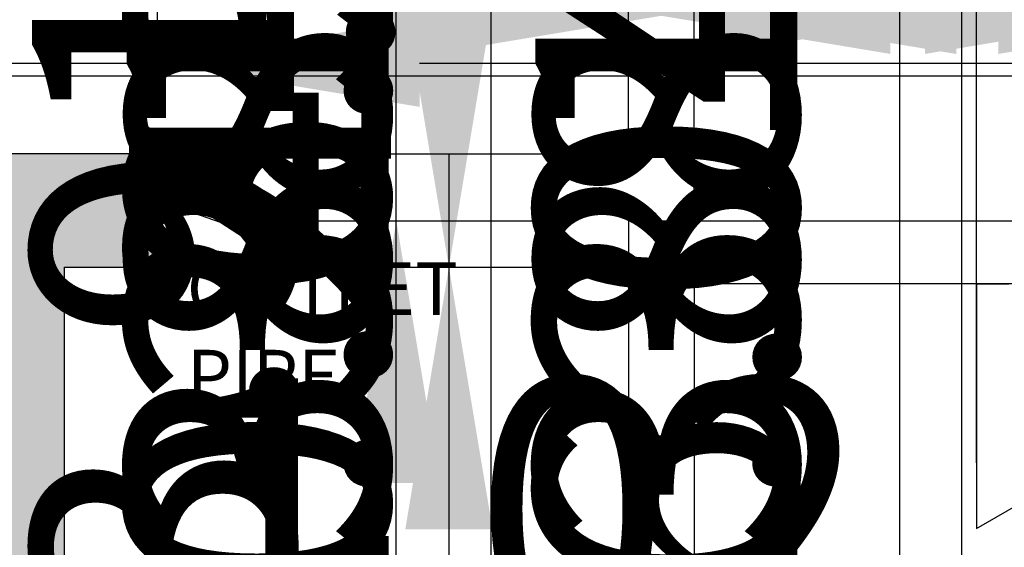
# Model space of a CAD drawing. Units: metres. Extents: x 782 to 1487, y 1262 to 7446.
# Tile 9 of 25: x 830.694 to 840.091, y 1279.507 to 1284.539. Entities that reach past the tile are written whole.
import ezdxf

# ---------------------------------------------------------------- set-up
doc = ezdxf.new("R2010")
doc.units = ezdxf.units.M
for name, color, linetype, lineweight in [('A-ANNO-DIMS', 2, 'Continuous', 18), ('A-ANNO-TEXT', 3, 'Continuous', 18), ('A-DETL', 7, 'Continuous', 25), ('A-DETL-PATT', 9, 'Continuous', 13)]:
    doc.layers.add(name, color=color, linetype=linetype, lineweight=lineweight)
doc.styles.get("Standard").update_dxf_attribs({"font": 'arial.ttf'})
doc.dimstyles.new('ISO-25', dxfattribs={"dimtxt": 2.5, "dimasz": 2.5, "dimexe": 1.25, "dimexo": 0.625, "dimtad": 1, "dimtxsty": 'Standard', "dimcen": 2.5, "dimadec": 0, "dimazin": 0, "dimtfac": 1, "dimtmove": 0, "dimatfit": 3, "dimfxl": 1, "dimarcsym": 0})

# ---------------------------------------------------------------- blocks, each defined once
blk = doc.blocks.new('*D10')
at = {"layer": 'A-ANNO-DIMS', "color": 0, "lineweight": -2, "transparency": 16777216}
for p, q in [((825.7296, 1277.5266), (825.7296, 1276.1659)), ((826.7525, 1277.552), (826.7525, 1276.1659)), ((823.2296, 1277.4159), (820.7296, 1277.4159)), ((825.7296, 1277.4159), (826.7525, 1277.4159)), ((829.2525, 1277.4159), (839.2355, 1277.4159))]:
    blk.add_line(p, q, dxfattribs=at)
at = {"layer": 'A-ANNO-DIMS', "color": 0, "transparency": 16777216}
for points in [[(823.2296, 1277.8326), (823.2296, 1276.9992), (825.7296, 1277.4159)], [(829.2525, 1277.8326), (829.2525, 1276.9992), (826.7525, 1277.4159)]]:
    blk.add_solid(points, dxfattribs=at)
at = {"layer": 'Defpoints', "color": 0, "transparency": 16777216}
for p in [(825.7296, 1278.1516), (826.7525, 1278.177), (826.7525, 1277.4159)]:
    blk.add_point(p, dxfattribs=at)
at = {"layer": 'A-ANNO-DIMS', "color": 0, "transparency": 16777216, "insert": (835.494, 1279.5433), "char_height": 2.5, "attachment_point": 5}
blk.add_mtext('1,02', dxfattribs=at)
blk = doc.blocks.new('*D89')
at = {"layer": 'A-ANNO-DIMS', "color": 0, "lineweight": -2, "transparency": 16777216}
for p, q in [((835.1905, 1302.8378), (835.1905, 1305.3378)), ((833.0381, 1300.3378), (836.4405, 1300.3378)), ((835.1905, 1300.3378), (835.1905, 1296.196)), ((833.0375, 1296.196), (836.4405, 1296.196)), ((835.1905, 1293.696), (835.1905, 1281.4347))]:
    blk.add_line(p, q, dxfattribs=at)
at = {"layer": 'A-ANNO-DIMS', "color": 0, "transparency": 16777216}
for points in [[(834.7738, 1302.8378), (835.6071, 1302.8378), (835.1905, 1300.3378)], [(834.7738, 1293.696), (835.6071, 1293.696), (835.1905, 1296.196)]]:
    blk.add_solid(points, dxfattribs=at)
at = {"layer": 'Defpoints', "color": 0, "transparency": 16777216}
for p in [(832.4131, 1300.3378), (832.4125, 1296.196), (835.1905, 1296.196)]:
    blk.add_point(p, dxfattribs=at)
at = {"layer": 'A-ANNO-DIMS', "color": 0, "transparency": 16777216, "insert": (833.3103, 1286.3153), "char_height": 2.5, "attachment_point": 5, "rotation": 90}
blk.add_mtext('4.142', dxfattribs=at)
blk = doc.blocks.new('*D90')
at = {"layer": 'A-ANNO-DIMS', "color": 0, "lineweight": -2, "transparency": 16777216}
for p, q in [((835.1905, 1298.696), (835.1905, 1301.196)), ((833.0375, 1296.196), (836.4405, 1296.196)), ((835.1905, 1296.196), (835.1905, 1293.6994)), ((833.0375, 1293.6994), (836.4405, 1293.6994)), ((835.1905, 1291.1994), (835.1905, 1280.9214))]:
    blk.add_line(p, q, dxfattribs=at)
at = {"layer": 'A-ANNO-DIMS', "color": 0, "transparency": 16777216}
for points in [[(834.7738, 1298.696), (835.6071, 1298.696), (835.1905, 1296.196)], [(834.7738, 1291.1994), (835.6071, 1291.1994), (835.1905, 1293.6994)]]:
    blk.add_solid(points, dxfattribs=at)
at = {"layer": 'Defpoints', "color": 0, "transparency": 16777216}
for p in [(832.4125, 1296.196), (832.4125, 1293.6994), (835.1905, 1293.6994)]:
    blk.add_point(p, dxfattribs=at)
at = {"layer": 'A-ANNO-DIMS', "color": 0, "transparency": 16777216, "insert": (833.289, 1284.8104), "char_height": 2.5, "attachment_point": 5, "rotation": 90}
blk.add_mtext('2.50', dxfattribs=at)
blk = doc.blocks.new('*D91')
at = {"layer": 'A-ANNO-DIMS', "color": 0, "lineweight": -2, "transparency": 16777216}
for p, q in [((835.1905, 1296.1994), (835.1905, 1298.6994)), ((833.0375, 1293.6994), (836.4405, 1293.6994)), ((835.1905, 1293.6994), (835.1905, 1293.0674)), ((833.0375, 1293.0674), (836.4405, 1293.0674)), ((835.1905, 1290.5674), (835.1905, 1278.4068))]:
    blk.add_line(p, q, dxfattribs=at)
at = {"layer": 'A-ANNO-DIMS', "color": 0, "transparency": 16777216}
for points in [[(834.7738, 1296.1994), (835.6071, 1296.1994), (835.1905, 1293.6994)], [(834.7738, 1290.5674), (835.6071, 1290.5674), (835.1905, 1293.0674)]]:
    blk.add_solid(points, dxfattribs=at)
at = {"layer": 'Defpoints', "color": 0, "transparency": 16777216}
for p in [(832.4125, 1293.6994), (832.4125, 1293.0674), (835.1905, 1293.0674)]:
    blk.add_point(p, dxfattribs=at)
at = {"layer": 'A-ANNO-DIMS', "color": 0, "transparency": 16777216, "insert": (833.2882, 1283.2371), "char_height": 2.5, "attachment_point": 5, "rotation": 90}
blk.add_mtext('0.632', dxfattribs=at)
blk = doc.blocks.new('*D92')
at = {"layer": 'A-ANNO-DIMS', "color": 0, "lineweight": -2, "transparency": 16777216}
for p, q in [((835.1905, 1295.5674), (835.1905, 1298.0674)), ((831.3406, 1293.0674), (836.4405, 1293.0674)), ((835.1905, 1293.0674), (835.1905, 1291.6863)), ((831.3406, 1291.6863), (836.4405, 1291.6863)), ((835.1905, 1289.1863), (835.1905, 1277.7181))]:
    blk.add_line(p, q, dxfattribs=at)
at = {"layer": 'A-ANNO-DIMS', "color": 0, "transparency": 16777216}
for points in [[(834.7738, 1295.5674), (835.6071, 1295.5674), (835.1905, 1293.0674)], [(834.7738, 1289.1863), (835.6071, 1289.1863), (835.1905, 1291.6863)]]:
    blk.add_solid(points, dxfattribs=at)
at = {"layer": 'Defpoints', "color": 0, "transparency": 16777216}
for p in [(830.7156, 1293.0674), (830.7156, 1291.6863), (835.1905, 1291.6863)]:
    blk.add_point(p, dxfattribs=at)
at = {"layer": 'A-ANNO-DIMS', "color": 0, "transparency": 16777216, "insert": (833.2882, 1282.2022), "char_height": 2.5, "attachment_point": 5, "rotation": 90}
blk.add_mtext('1.381', dxfattribs=at)
blk = doc.blocks.new('*D93')
at = {"layer": 'A-ANNO-DIMS', "color": 0, "lineweight": -2, "transparency": 16777216}
for p, q in [((835.1905, 1294.1863), (835.1905, 1296.6863)), ((831.3406, 1291.6863), (836.4405, 1291.6863)), ((835.1905, 1291.6863), (835.1905, 1290.3053)), ((831.3406, 1290.3053), (836.4405, 1290.3053)), ((835.1905, 1287.8053), (835.1905, 1276.337))]:
    blk.add_line(p, q, dxfattribs=at)
at = {"layer": 'A-ANNO-DIMS', "color": 0, "transparency": 16777216}
for points in [[(834.7738, 1294.1863), (835.6071, 1294.1863), (835.1905, 1291.6863)], [(834.7738, 1287.8053), (835.6071, 1287.8053), (835.1905, 1290.3053)]]:
    blk.add_solid(points, dxfattribs=at)
at = {"layer": 'Defpoints', "color": 0, "transparency": 16777216}
for p in [(830.7156, 1291.6863), (830.7156, 1290.3053), (835.1905, 1290.3053)]:
    blk.add_point(p, dxfattribs=at)
at = {"layer": 'A-ANNO-DIMS', "color": 0, "transparency": 16777216, "insert": (833.2882, 1280.8211), "char_height": 2.5, "attachment_point": 5, "rotation": 90}
blk.add_mtext('1.381', dxfattribs=at)
blk = doc.blocks.new('*D112')
at = {"layer": 'A-ANNO-DIMS', "color": 0, "lineweight": -2, "transparency": 16777216}
for p, q in [((839.0913, 1301.6153), (839.0913, 1304.1153)), ((839.4663, 1299.1153), (837.8413, 1299.1153)), ((839.0913, 1299.1153), (839.0913, 1293.0674)), ((839.4663, 1293.0674), (837.8413, 1293.0674)), ((839.0913, 1290.5674), (839.0913, 1278.3624))]:
    blk.add_line(p, q, dxfattribs=at)
at = {"layer": 'A-ANNO-DIMS', "color": 0, "transparency": 16777216}
for points in [[(838.6746, 1301.6153), (839.508, 1301.6153), (839.0913, 1299.1153)], [(838.6746, 1290.5674), (839.508, 1290.5674), (839.0913, 1293.0674)]]:
    blk.add_solid(points, dxfattribs=at)
at = {"layer": 'Defpoints', "color": 0, "transparency": 16777216}
for p in [(840.0913, 1299.1153), (839.0913, 1293.0674), (840.0913, 1293.0674)]:
    blk.add_point(p, dxfattribs=at)
at = {"layer": 'A-ANNO-DIMS', "color": 0, "transparency": 16777216, "insert": (837.1899, 1283.2149), "char_height": 2.5, "attachment_point": 5, "rotation": 90}
blk.add_mtext('6.048', dxfattribs=at)
blk = doc.blocks.new('*D113')
at = {"layer": 'A-ANNO-DIMS', "color": 0, "lineweight": -2, "transparency": 16777216}
for p, q in [((839.0913, 1295.5674), (839.0913, 1298.0674)), ((839.4663, 1293.0674), (837.8413, 1293.0674)), ((839.0913, 1293.0674), (839.0913, 1291.6863)), ((839.4663, 1291.6863), (837.8413, 1291.6863)), ((839.0913, 1289.1863), (839.0913, 1277.7181))]:
    blk.add_line(p, q, dxfattribs=at)
at = {"layer": 'A-ANNO-DIMS', "color": 0, "transparency": 16777216}
for points in [[(838.6746, 1295.5674), (839.508, 1295.5674), (839.0913, 1293.0674)], [(838.6746, 1289.1863), (839.508, 1289.1863), (839.0913, 1291.6863)]]:
    blk.add_solid(points, dxfattribs=at)
at = {"layer": 'Defpoints', "color": 0, "transparency": 16777216}
for p in [(840.0913, 1293.0674), (839.0913, 1291.6863), (840.0913, 1291.6863)]:
    blk.add_point(p, dxfattribs=at)
at = {"layer": 'A-ANNO-DIMS', "color": 0, "transparency": 16777216, "insert": (837.189, 1282.2022), "char_height": 2.5, "attachment_point": 5, "rotation": 90}
blk.add_mtext('1.381', dxfattribs=at)
blk = doc.blocks.new('*D114')
at = {"layer": 'A-ANNO-DIMS', "color": 0, "lineweight": -2, "transparency": 16777216}
for p, q in [((839.0913, 1294.1863), (839.0913, 1296.6863)), ((839.4663, 1291.6863), (837.8413, 1291.6863)), ((839.0913, 1291.6863), (839.0913, 1290.3053)), ((839.4663, 1290.3053), (837.8413, 1290.3053)), ((839.0913, 1287.8053), (839.0913, 1276.337))]:
    blk.add_line(p, q, dxfattribs=at)
at = {"layer": 'A-ANNO-DIMS', "color": 0, "transparency": 16777216}
for points in [[(838.6746, 1294.1863), (839.508, 1294.1863), (839.0913, 1291.6863)], [(838.6746, 1287.8053), (839.508, 1287.8053), (839.0913, 1290.3053)]]:
    blk.add_solid(points, dxfattribs=at)
at = {"layer": 'Defpoints', "color": 0, "transparency": 16777216}
for p in [(840.0913, 1291.6863), (839.0913, 1290.3053), (840.0913, 1290.3053)]:
    blk.add_point(p, dxfattribs=at)
at = {"layer": 'A-ANNO-DIMS', "color": 0, "transparency": 16777216, "insert": (837.189, 1280.8211), "char_height": 2.5, "attachment_point": 5, "rotation": 90}
blk.add_mtext('1.381', dxfattribs=at)
blk = doc.blocks.new('*D151')
at = {"layer": 'A-ANNO-DIMS', "color": 0, "lineweight": -2, "transparency": 16777216}
for p, q in [((839.686, 1273.6942), (839.686, 1285.8791)), ((841.835, 1273.6942), (841.835, 1285.8791)), ((837.186, 1284.6291), (834.686, 1284.6291)), ((839.686, 1284.6291), (841.835, 1284.6291)), ((844.335, 1284.6291), (856.569, 1284.6291))]:
    blk.add_line(p, q, dxfattribs=at)
at = {"layer": 'A-ANNO-DIMS', "color": 0, "transparency": 16777216}
for points in [[(837.186, 1285.0458), (837.186, 1284.2125), (839.686, 1284.6291)], [(844.335, 1285.0458), (844.335, 1284.2125), (841.835, 1284.6291)]]:
    blk.add_solid(points, dxfattribs=at)
at = {"layer": 'Defpoints', "color": 0, "transparency": 16777216}
for p in [(841.835, 1284.6291), (839.686, 1273.0692), (841.835, 1273.0692)]:
    blk.add_point(p, dxfattribs=at)
at = {"layer": 'A-ANNO-DIMS', "color": 0, "transparency": 16777216, "insert": (851.702, 1286.5306), "char_height": 2.5, "attachment_point": 5}
blk.add_mtext('2.149', dxfattribs=at)
blk = doc.blocks.new('*D152')
at = {"layer": 'A-ANNO-DIMS', "color": 0, "lineweight": -2, "transparency": 16777216}
for p, q in [((841.835, 1273.6942), (841.835, 1285.8791)), ((842.5333, 1273.6783), (842.5333, 1285.8791)), ((839.335, 1284.6291), (836.835, 1284.6291)), ((841.835, 1284.6291), (842.5333, 1284.6291)), ((845.0333, 1284.6291), (855.2686, 1284.6291))]:
    blk.add_line(p, q, dxfattribs=at)
at = {"layer": 'A-ANNO-DIMS', "color": 0, "transparency": 16777216}
for points in [[(839.335, 1285.0458), (839.335, 1284.2125), (841.835, 1284.6291)], [(845.0333, 1285.0458), (845.0333, 1284.2125), (842.5333, 1284.6291)]]:
    blk.add_solid(points, dxfattribs=at)
at = {"layer": 'Defpoints', "color": 0, "transparency": 16777216}
for p in [(842.5333, 1284.6291), (841.835, 1273.0692), (842.5333, 1273.0533)]:
    blk.add_point(p, dxfattribs=at)
at = {"layer": 'A-ANNO-DIMS', "color": 0, "transparency": 16777216, "insert": (851.4009, 1286.5306), "char_height": 2.5, "attachment_point": 5}
blk.add_mtext('0.70', dxfattribs=at)
blk = doc.blocks.new('*D153')
at = {"layer": 'A-ANNO-DIMS', "color": 0, "lineweight": -2, "transparency": 16777216}
for p, q in [((842.5333, 1273.6783), (842.5333, 1285.8791)), ((844.6687, 1273.6976), (844.6687, 1285.8791)), ((840.0333, 1284.6291), (837.5333, 1284.6291)), ((842.5333, 1284.6291), (844.6687, 1284.6291)), ((847.1687, 1284.6291), (857.445, 1284.6291))]:
    blk.add_line(p, q, dxfattribs=at)
at = {"layer": 'A-ANNO-DIMS', "color": 0, "transparency": 16777216}
for points in [[(840.0333, 1285.0458), (840.0333, 1284.2125), (842.5333, 1284.6291)], [(847.1687, 1285.0458), (847.1687, 1284.2125), (844.6687, 1284.6291)]]:
    blk.add_solid(points, dxfattribs=at)
at = {"layer": 'Defpoints', "color": 0, "transparency": 16777216}
for p in [(844.6687, 1284.6291), (842.5333, 1273.0533), (844.6687, 1273.0726)]:
    blk.add_point(p, dxfattribs=at)
at = {"layer": 'A-ANNO-DIMS', "color": 0, "transparency": 16777216, "insert": (853.5568, 1286.5093), "char_height": 2.5, "attachment_point": 5}
blk.add_mtext('2.14', dxfattribs=at)
blk = doc.blocks.new('*D154')
at = {"layer": 'A-ANNO-DIMS', "color": 0, "lineweight": -2, "transparency": 16777216}
for p, q in [((834.2886, 1275.5562), (834.2886, 1287.7305)), ((836.1342, 1273.0562), (833.0386, 1273.0562)), ((834.2886, 1269.1422), (834.2886, 1273.0562)), ((836.1187, 1269.1422), (833.0386, 1269.1422)), ((834.2886, 1266.6422), (834.2886, 1264.1422))]:
    blk.add_line(p, q, dxfattribs=at)
at = {"layer": 'A-ANNO-DIMS', "color": 0, "transparency": 16777216}
for points in [[(833.8719, 1275.5562), (834.7052, 1275.5562), (834.2886, 1273.0562)], [(833.8719, 1266.6422), (834.7052, 1266.6422), (834.2886, 1269.1422)]]:
    blk.add_solid(points, dxfattribs=at)
at = {"layer": 'Defpoints', "color": 0, "transparency": 16777216}
for p in [(834.2886, 1273.0562), (836.7592, 1273.0562), (836.7437, 1269.1422)]:
    blk.add_point(p, dxfattribs=at)
at = {"layer": 'A-ANNO-DIMS', "color": 0, "transparency": 16777216, "insert": (832.3863, 1282.8934), "char_height": 2.5, "attachment_point": 5, "rotation": 90}
blk.add_mtext('3.914', dxfattribs=at)
blk = doc.blocks.new('*D156')
at = {"layer": 'A-ANNO-DIMS', "color": 0, "lineweight": -2, "transparency": 16777216}
for p, q in [((836.5033, 1283.244), (836.5033, 1285.8791)), ((846.1759, 1283.244), (846.1759, 1285.8791)), ((839.0033, 1284.6291), (843.6759, 1284.6291)), ((846.1759, 1284.6291), (858.3621, 1284.6291))]:
    blk.add_line(p, q, dxfattribs=at)
at = {"layer": 'A-ANNO-DIMS', "color": 0, "transparency": 16777216}
for points in [[(839.0033, 1285.0458), (839.0033, 1284.2125), (836.5033, 1284.6291)], [(843.6759, 1285.0458), (843.6759, 1284.2125), (846.1759, 1284.6291)]]:
    blk.add_solid(points, dxfattribs=at)
at = {"layer": 'Defpoints', "color": 0, "transparency": 16777216}
for p in [(846.1759, 1284.6291), (836.5033, 1282.619), (846.1759, 1282.619)]:
    blk.add_point(p, dxfattribs=at)
at = {"layer": 'A-ANNO-DIMS', "color": 0, "transparency": 16777216, "insert": (853.519, 1286.5314), "char_height": 2.5, "attachment_point": 5}
blk.add_mtext('9.673', dxfattribs=at)
blk = doc.blocks.new('*D157')
at = {"layer": 'A-ANNO-DIMS', "color": 0, "lineweight": -2, "transparency": 16777216}
for p, q in [((834.2886, 1282.619), (834.2886, 1294.8189)), ((835.8783, 1282.619), (833.0386, 1282.619)), ((834.2886, 1278.7022), (834.2886, 1280.119)), ((835.8783, 1276.2022), (833.0386, 1276.2022))]:
    blk.add_line(p, q, dxfattribs=at)
at = {"layer": 'A-ANNO-DIMS', "color": 0, "transparency": 16777216}
for points in [[(833.8719, 1280.119), (834.7052, 1280.119), (834.2886, 1282.619)], [(833.8719, 1278.7022), (834.7052, 1278.7022), (834.2886, 1276.2022)]]:
    blk.add_solid(points, dxfattribs=at)
at = {"layer": 'Defpoints', "color": 0, "transparency": 16777216}
for p in [(834.2886, 1282.619), (836.5033, 1282.619), (836.5033, 1276.2022)]:
    blk.add_point(p, dxfattribs=at)
at = {"layer": 'A-ANNO-DIMS', "color": 0, "transparency": 16777216, "insert": (832.3871, 1289.9689), "char_height": 2.5, "attachment_point": 5, "rotation": 90}
blk.add_mtext('6.417', dxfattribs=at)
blk = doc.blocks.new('*D158')
at = {"layer": 'A-ANNO-DIMS', "color": 0, "lineweight": -2, "transparency": 16777216}
for p, q in [((836.5033, 1283.244), (836.5033, 1285.8791)), ((837.1321, 1282.6436), (837.1321, 1285.8791)), ((834.0033, 1284.6291), (831.5033, 1284.6291)), ((836.5033, 1284.6291), (837.1321, 1284.6291)), ((839.6321, 1284.6291), (849.876, 1284.6291))]:
    blk.add_line(p, q, dxfattribs=at)
at = {"layer": 'A-ANNO-DIMS', "color": 0, "transparency": 16777216}
for points in [[(834.0033, 1285.0458), (834.0033, 1284.2125), (836.5033, 1284.6291)], [(839.6321, 1285.0458), (839.6321, 1284.2125), (837.1321, 1284.6291)]]:
    blk.add_solid(points, dxfattribs=at)
at = {"layer": 'Defpoints', "color": 0, "transparency": 16777216}
for p in [(837.1321, 1284.6291), (836.5033, 1282.619), (837.1321, 1282.0186)]:
    blk.add_point(p, dxfattribs=at)
at = {"layer": 'A-ANNO-DIMS', "color": 0, "transparency": 16777216, "insert": (846.004, 1286.5314), "char_height": 2.5, "attachment_point": 5}
blk.add_mtext('0.63', dxfattribs=at)
blk = doc.blocks.new('*D159')
at = {"layer": 'A-ANNO-DIMS', "color": 0, "lineweight": -2, "transparency": 16777216}
for p, q in [((837.1321, 1282.6436), (837.1321, 1285.8791)), ((839.8262, 1282.6436), (839.8262, 1285.8791)), ((834.6321, 1284.6291), (832.1321, 1284.6291)), ((837.1321, 1284.6291), (839.8262, 1284.6291)), ((842.3262, 1284.6291), (854.5449, 1284.6291))]:
    blk.add_line(p, q, dxfattribs=at)
at = {"layer": 'A-ANNO-DIMS', "color": 0, "transparency": 16777216}
for points in [[(834.6321, 1285.0458), (834.6321, 1284.2125), (837.1321, 1284.6291)], [(842.3262, 1285.0458), (842.3262, 1284.2125), (839.8262, 1284.6291)]]:
    blk.add_solid(points, dxfattribs=at)
at = {"layer": 'Defpoints', "color": 0, "transparency": 16777216}
for p in [(839.8262, 1284.6291), (837.1321, 1282.0186), (839.8262, 1282.0186)]:
    blk.add_point(p, dxfattribs=at)
at = {"layer": 'A-ANNO-DIMS', "color": 0, "transparency": 16777216, "insert": (849.6855, 1286.5306), "char_height": 2.5, "attachment_point": 5}
blk.add_mtext('2.694', dxfattribs=at)
blk = doc.blocks.new('*D160')
at = {"layer": 'A-ANNO-DIMS', "color": 0, "lineweight": -2, "transparency": 16777216}
for p, q in [((839.8262, 1280.3128), (839.8262, 1285.8791)), ((841.2554, 1280.4442), (841.2554, 1285.8791)), ((837.3262, 1284.6291), (834.8262, 1284.6291)), ((839.8262, 1284.6291), (841.2554, 1284.6291)), ((843.7554, 1284.6291), (853.764, 1284.6291))]:
    blk.add_line(p, q, dxfattribs=at)
at = {"layer": 'A-ANNO-DIMS', "color": 0, "transparency": 16777216}
for points in [[(837.3262, 1285.0458), (837.3262, 1284.2125), (839.8262, 1284.6291)], [(843.7554, 1285.0458), (843.7554, 1284.2125), (841.2554, 1284.6291)]]:
    blk.add_solid(points, dxfattribs=at)
at = {"layer": 'Defpoints', "color": 0, "transparency": 16777216}
for p in [(841.2554, 1284.6291), (841.2554, 1279.8192), (839.8262, 1279.6878)]:
    blk.add_point(p, dxfattribs=at)
at = {"layer": 'A-ANNO-DIMS', "color": 0, "transparency": 16777216, "insert": (850.0097, 1286.5314), "char_height": 2.5, "attachment_point": 5}
blk.add_mtext('1.43', dxfattribs=at)
blk = doc.blocks.new('*D165')
at = {"layer": 'A-ANNO-DIMS', "color": 0, "lineweight": -2, "transparency": 16777216}
for p, q in [((826.3877, 1283.8847), (826.3877, 1285.3747)), ((832.0105, 1283.8847), (832.0105, 1285.3747)), ((823.8877, 1284.1247), (821.3877, 1284.1247)), ((826.3877, 1284.1247), (832.0105, 1284.1247)), ((834.5105, 1284.1247), (846.6967, 1284.1247))]:
    blk.add_line(p, q, dxfattribs=at)
at = {"layer": 'A-ANNO-DIMS', "color": 0, "transparency": 16777216}
for points in [[(823.8877, 1284.5413), (823.8877, 1283.708), (826.3877, 1284.1247)], [(834.5105, 1284.5413), (834.5105, 1283.708), (832.0105, 1284.1247)]]:
    blk.add_solid(points, dxfattribs=at)
at = {"layer": 'Defpoints', "color": 0, "transparency": 16777216}
for p in [(832.0105, 1284.1247), (826.3877, 1283.2597), (832.0105, 1283.2597)]:
    blk.add_point(p, dxfattribs=at)
at = {"layer": 'A-ANNO-DIMS', "color": 0, "transparency": 16777216, "insert": (841.8536, 1286.027), "char_height": 2.5, "attachment_point": 5}
blk.add_mtext('5.623', dxfattribs=at)
blk = doc.blocks.new('*D167')
at = {"layer": 'A-ANNO-DIMS', "color": 0, "lineweight": -2, "transparency": 16777216}
for p, q in [((834.7907, 1285.7597), (834.7907, 1288.2597)), ((832.6355, 1283.2597), (836.0407, 1283.2597)), ((834.7907, 1283.2597), (834.7907, 1282.1784)), ((831.7457, 1282.1784), (836.0407, 1282.1784)), ((834.7907, 1279.6784), (834.7907, 1269.6648))]:
    blk.add_line(p, q, dxfattribs=at)
at = {"layer": 'A-ANNO-DIMS', "color": 0, "transparency": 16777216}
for points in [[(834.3741, 1285.7597), (835.2074, 1285.7597), (834.7907, 1283.2597)], [(834.3741, 1279.6784), (835.2074, 1279.6784), (834.7907, 1282.1784)]]:
    blk.add_solid(points, dxfattribs=at)
at = {"layer": 'Defpoints', "color": 0, "transparency": 16777216}
for p in [(832.0105, 1283.2597), (831.1207, 1282.1784), (834.7907, 1282.1784)]:
    blk.add_point(p, dxfattribs=at)
at = {"layer": 'A-ANNO-DIMS', "color": 0, "transparency": 16777216, "insert": (832.8893, 1273.4216), "char_height": 2.5, "attachment_point": 5, "rotation": 90}
blk.add_mtext('1.08', dxfattribs=at)
blk = doc.blocks.new('*D168')
at = {"layer": 'A-ANNO-DIMS', "color": 0, "lineweight": -2, "transparency": 16777216}
for p, q in [((834.7907, 1284.6784), (834.7907, 1287.1784)), ((831.7457, 1282.1784), (836.0407, 1282.1784)), ((834.7907, 1282.1784), (834.7907, 1279.1214)), ((831.7457, 1279.1214), (836.0407, 1279.1214)), ((834.7907, 1276.6214), (834.7907, 1264.4369))]:
    blk.add_line(p, q, dxfattribs=at)
at = {"layer": 'A-ANNO-DIMS', "color": 0, "transparency": 16777216}
for points in [[(834.3741, 1284.6784), (835.2074, 1284.6784), (834.7907, 1282.1784)], [(834.3741, 1276.6214), (835.2074, 1276.6214), (834.7907, 1279.1214)]]:
    blk.add_solid(points, dxfattribs=at)
at = {"layer": 'Defpoints', "color": 0, "transparency": 16777216}
for p in [(831.1207, 1282.1784), (831.1207, 1279.1214), (834.7907, 1279.1214)]:
    blk.add_point(p, dxfattribs=at)
at = {"layer": 'A-ANNO-DIMS', "color": 0, "transparency": 16777216, "insert": (832.8885, 1269.2791), "char_height": 2.5, "attachment_point": 5, "rotation": 90}
blk.add_mtext('3.057', dxfattribs=at)

msp = doc.modelspace()

# ---------------------------------------------------------------- hatches: boundary and pattern name
at = {"layer": 'A-DETL-PATT'}
h = msp.add_hatch(color=256, dxfattribs=at)
h.dxf.hatch_style = 1
h.paths.add_polyline_path([(831.1207, 1282.1784), (832.0105, 1282.1784), (832.0105, 1283.2597), (826.3877, 1283.2597), (826.3877, 1282.1784), (827.6538, 1282.1784), (827.6538, 1279.1214), (831.1207, 1279.1214)])
h.paths.add_polyline_path([(823.78, 1277.2166), (828.1675, 1277.2166), (828.1675, 1282.4262), (823.78, 1282.4262)], flags=9)
h = msp.add_hatch(color=256, dxfattribs=at)
h.dxf.hatch_style = 1
h.paths.add_polyline_path([(831.1207, 1282.1784), (832.0105, 1282.1784), (832.0105, 1283.2597), (826.3877, 1283.2597), (826.3877, 1282.1784), (827.6538, 1282.1784), (827.6538, 1279.1214), (831.1207, 1279.1214)])
h.paths.add_polyline_path([(823.78, 1277.2166), (828.1675, 1277.2166), (828.1675, 1282.4262), (823.78, 1282.4262)], flags=9)

# ---------------------------------------------------------------- linework, layer by layer
at = {"layer": 'A-DETL'}
for p, q in [((832.0105, 1283.2597), (826.3877, 1283.2597)), ((832.0105, 1282.1784), (832.0105, 1283.2597)), ((832.0105, 1282.7191), (832.2886, 1282.7191)), ((832.788, 1282.6769), (832.0105, 1282.7191)), ((832.2886, 1282.7191), (833.2348, 1282.39)), ((833.2348, 1282.6769), (832.788, 1282.6769)), ((833.2348, 1282.39), (833.2348, 1282.6769)), ((831.1207, 1279.1214), (831.1207, 1282.1784)), ((831.1207, 1282.1784), (832.0105, 1282.1784)), ((831.8427, 1282.1784), (832.0105, 1282.1784)), ((841.4362, 1282.0186), (839.8262, 1282.0186)), ((839.8262, 1282.0186), (839.8262, 1279.6878)), ((839.8262, 1282.0186), (840.1341, 1282.0186)), ((839.8262, 1279.6878), (840.8283, 1280.2623))]:
    msp.add_line(p, q, dxfattribs=at)
for points in [[(823.6278, 1284.0012), (823.6278, 1266.59), (847.1334, 1266.59), (847.1334, 1284.0012)], [(836.5033, 1282.619), (836.5033, 1276.2022), (846.1759, 1276.2022), (846.1759, 1282.619)], [(837.1321, 1282.0186), (837.1321, 1276.6513), (845.7402, 1276.6513), (845.7402, 1282.0186)]]:
    msp.add_lwpolyline(points, close=True, dxfattribs=at)

# ---------------------------------------------------------------- texts
at = {"layer": 'A-ANNO-TEXT', "insert": (832.2886, 1283.0579), "char_height": 0.5, "attachment_point": 1}
msp.add_mtext_dynamic_manual_height_columns('\\POUTLET PIPE', width=2.466436, gutter_width=12.5, heights=[0], dxfattribs=at)

# ---------------------------------------------------------------- dimensions: what is measured, and where the dimension line sits
at = {"layer": 'A-ANNO-DIMS'}
for base, p1, p2, override, picture, middle in [((835.1905, 1296.196), (832.4131, 1300.3378), (832.4125, 1296.196), {"dimdec": 3, "dimlfac": 1, "dimrnd": 0, "dimzin": 0, "dimdsep": 46, "dimlunit": 2}, '*D89', (833.3103, 1286.3153)), ((839.0913, 1293.0674), (840.0913, 1299.1153), (840.0913, 1293.0674), {"dimdec": 3, "dimlfac": 1, "dimrnd": 0, "dimzin": 0, "dimdsep": 46, "dimlunit": 2}, '*D112', (837.1899, 1283.2149)), ((835.1905, 1293.6994), (832.4125, 1296.196), (832.4125, 1293.6994), {"dimdec": 2, "dimlfac": 1, "dimrnd": 0, "dimzin": 0, "dimdsep": 46, "dimlunit": 2}, '*D90', (833.289, 1284.8104)), ((835.1905, 1293.0674), (832.4125, 1293.6994), (832.4125, 1293.0674), {"dimdec": 3, "dimlfac": 1, "dimrnd": 0, "dimzin": 0, "dimdsep": 46, "dimlunit": 2}, '*D91', (833.2882, 1283.2371)), ((835.1905, 1291.6863), (830.7156, 1293.0674), (830.7156, 1291.6863), {"dimdec": 3, "dimlfac": 1, "dimrnd": 0, "dimzin": 0, "dimdsep": 46, "dimlunit": 2}, '*D92', (833.2882, 1282.2022)), ((839.0913, 1291.6863), (840.0913, 1293.0674), (840.0913, 1291.6863), {"dimdec": 3, "dimlfac": 1, "dimrnd": 0, "dimzin": 0, "dimdsep": 46, "dimlunit": 2}, '*D113', (837.189, 1282.2022)), ((835.1905, 1290.3053), (830.7156, 1291.6863), (830.7156, 1290.3053), {"dimdec": 3, "dimlfac": 1, "dimrnd": 0, "dimzin": 0, "dimdsep": 46, "dimlunit": 2}, '*D93', (833.2882, 1280.8211)), ((839.0913, 1290.3053), (840.0913, 1291.6863), (840.0913, 1290.3053), {"dimdec": 3, "dimlfac": 1, "dimrnd": 0, "dimzin": 0, "dimdsep": 46, "dimlunit": 2}, '*D114', (837.189, 1280.8211)), ((834.2886, 1282.619), (836.5033, 1276.2022), (836.5033, 1282.619), {"dimdec": 3, "dimlfac": 1, "dimrnd": 0, "dimzin": 0, "dimdsep": 46, "dimlunit": 2}, '*D157', (832.3871, 1289.9689)), ((834.7907, 1282.1784), (832.0105, 1283.2597), (831.1207, 1282.1784), {"dimdec": 2, "dimlfac": 1, "dimrnd": 0, "dimzin": 0, "dimdsep": 46, "dimlunit": 2}, '*D167', (832.8893, 1273.4216)), ((834.2886, 1273.0562), (836.7437, 1269.1422), (836.7592, 1273.0562), {"dimdec": 3, "dimlfac": 1, "dimrnd": 0, "dimzin": 0, "dimdsep": 46, "dimlunit": 2}, '*D154', (832.3863, 1282.8934)), ((834.7907, 1279.1214), (831.1207, 1282.1784), (831.1207, 1279.1214), {"dimdec": 3, "dimlfac": 1, "dimrnd": 0, "dimzin": 0, "dimdsep": 46, "dimlunit": 2}, '*D168', (832.8885, 1269.2791))]:
    dim = msp.add_linear_dim(base=base, p1=p1, p2=p2, angle=90, dimstyle='ISO-25', override=override, dxfattribs=at)
    dim.commit()
    dim.dimension.update_dxf_attribs({"geometry": picture, "text_midpoint": middle})
for base, p1, p2, override, picture, middle in [((837.1321, 1284.6291), (836.5033, 1282.619), (837.1321, 1282.0186), {"dimdec": 2, "dimlfac": 1, "dimrnd": 0, "dimzin": 0, "dimdsep": 46, "dimlunit": 2}, '*D158', (846.004, 1286.5314)), ((839.8262, 1284.6291), (837.1321, 1282.0186), (839.8262, 1282.0186), {"dimdec": 3, "dimlfac": 1, "dimrnd": 0, "dimzin": 0, "dimdsep": 46, "dimlunit": 2}, '*D159', (849.6855, 1286.5306)), ((841.835, 1284.6291), (839.686, 1273.0692), (841.835, 1273.0692), {"dimdec": 3, "dimlfac": 1, "dimrnd": 0, "dimzin": 0, "dimdsep": 46, "dimlunit": 2}, '*D151', (851.702, 1286.5306)), ((841.2554, 1284.6291), (839.8262, 1279.6878), (841.2554, 1279.8192), {"dimdec": 2, "dimlfac": 1, "dimrnd": 0, "dimzin": 0, "dimdsep": 46, "dimlunit": 2}, '*D160', (850.0097, 1286.5314)), ((846.1759, 1284.6291), (836.5033, 1282.619), (846.1759, 1282.619), {"dimdec": 3, "dimlfac": 1, "dimrnd": 0, "dimzin": 0, "dimdsep": 46, "dimlunit": 2}, '*D156', (853.519, 1286.5314)), ((842.5333, 1284.6291), (841.835, 1273.0692), (842.5333, 1273.0533), {"dimdec": 2, "dimlfac": 1, "dimrnd": 0, "dimzin": 0, "dimdsep": 46, "dimlunit": 2}, '*D152', (851.4009, 1286.5306)), ((844.6687, 1284.6291), (842.5333, 1273.0533), (844.6687, 1273.0726), {"dimdec": 2, "dimlfac": 1, "dimrnd": 0, "dimzin": 0, "dimdsep": 46, "dimlunit": 2}, '*D153', (853.5568, 1286.5093)), ((832.0105, 1284.1247), (826.3877, 1283.2597), (832.0105, 1283.2597), {"dimdec": 3, "dimlfac": 1, "dimrnd": 0, "dimzin": 0, "dimdsep": 46, "dimlunit": 2}, '*D165', (841.8536, 1286.027))]:
    dim = msp.add_linear_dim(base=base, p1=p1, p2=p2, dimstyle='ISO-25', override=override, dxfattribs=at)
    dim.commit()
    dim.dimension.update_dxf_attribs({"geometry": picture, "text_midpoint": middle})
dim = msp.add_linear_dim(base=(826.7525, 1277.4159), p1=(825.7296, 1278.1516), p2=(826.7525, 1278.177), dimstyle='ISO-25', override={"dimclrd": 0, "dimclre": 0, "dimclrt": 0}, dxfattribs=at)
dim.commit()
dim.dimension.update_dxf_attribs({"geometry": '*D10', "text_midpoint": (835.494, 1277.4159), "dimtype": 160})

doc.saveas('drawing.dxf')
